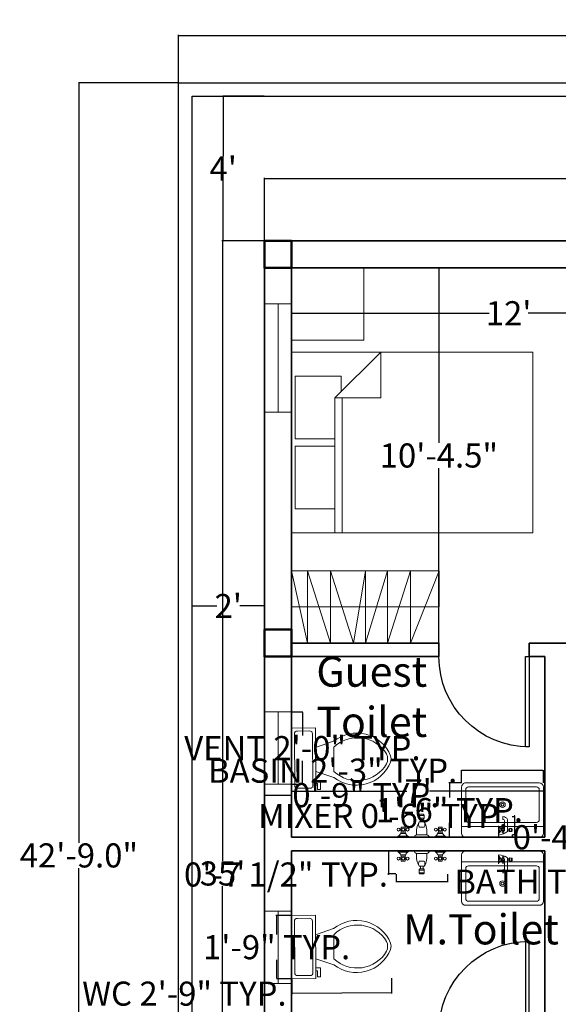
# Model space of a CAD drawing. Units: inches. Extents: x 20414 to 21627, y 49019 to 50314.
# Tile 6 of 10: x 20416 to 20594, y 49988 to 50314. Entities that reach past the tile are written whole.
import ezdxf

# ---------------------------------------------------------------- set-up
doc = ezdxf.new("R2010")
doc.units = ezdxf.units.IN
for name, color, linetype, lineweight in [('A-ANNO-DIMS', 7, 'Continuous', 18), ('A-AREA-IDEN', 7, 'Continuous', 18), ('A-FLOR-CASE', 2, 'Continuous', 18), ('C-PROP', 6, 'Continuous', 25), ('columns', 1, 'Continuous', 50), ('doors', 3, 'Continuous', 25), ('furniture', 2, 'Continuous', 18), ('plumbing', 1, 'Continuous', 18), ('walls', 6, 'Continuous', 35), ('windows', 3, 'Continuous', 18)]:
    doc.layers.add(name, color=color, linetype=linetype, lineweight=lineweight)
doc.styles.get("Standard").update_dxf_attribs({"font": 'arial.ttf'})
doc.dimstyles.get("Standard").update_dxf_attribs({"dimtxt": 8, "dimasz": 0.18, "dimexe": 0.18, "dimexo": 0.0625, "dimgap": 0.09, "dimtad": 0, "dimtih": 1, "dimtoh": 1, "dimdec": 1, "dimzin": 0, "dimdsep": 46, "dimlunit": 3, "dimtxsty": 'Standard', "dimcen": 0.09, "dimadec": 0, "dimazin": 0, "dimtfac": 1, "dimtdec": 1, "dimtofl": 0, "dimtmove": 0, "dimatfit": 3, "dimfxl": 1, "dimtolj": 1, "dimtzin": 0, "dimarcsym": 0})

# ---------------------------------------------------------------- blocks, each defined once
blk = doc.blocks.new('Bed - Queen')
for p, q in [((0, -80.00003), (0, 0)), ((0, 0), (59.99999, 0)), ((59.99999, 0), (59.99999, -80.00003)), ((7.99999, -1.2), (28.79998, -1.2)), ((7.99999, -14.4), (7.99999, -1.2)), ((28.79998, -1.2), (28.79998, -14.4)), ((31.19999, -1.2), (51.99999, -1.2)), ((31.19999, -14.4), (31.19999, -1.2)), ((51.99999, -1.2), (51.99999, -16.4)), ((0, -14.4), (44.8, -14.4)), ((59.99999, -29.6), (44.8, -14.4)), ((44.8, -14.4), (44.8, -29.6)), ((44.8, -16.8), (0, -16.8)), ((51.99999, -16.4), (46.79936, -16.4)), ((44.8, -29.6), (59.99999, -29.6)), ((59.99999, -80.00003), (0, -80.00003))]:
    blk.add_line(p, q)
blk = doc.blocks.new('Toilet - top')
for p, q in [((9.5, -6), (9.5, -2)), ((-10, -8.5), (-8, -8.5)), ((-10, -9.5), (-10, -8.5)), ((-7, -9.5), (-10, -9.5)), ((-8, -8.5), (-8, -8)), ((-7, -8), (-7, -9.5)), ((-4, -8), (-6, -14)), ((4, -8), (6, -14)), ((4, -14), (-4, -14))]:
    blk.add_line(p, q)
blk.add_lwpolyline([(10.5, -8), (10.5, 0), (-10.5, 0), (-10.5, -8)], close=True)
for points in [[(-9.5, -2), (-9.5, -6)], [(8.5, -1), (-8.5, -1)], [(-8.5, -7), (8.5, -7)]]:
    blk.add_lwpolyline(points)
for centre, radius, start, end in [((-8.62, -1.88), 0.884, 81.8699, 188.1301), ((8.62, -1.88), 0.884, 351.8699, 98.1301), ((-8.62, -6.12), 0.884, 171.8699, 278.1301), ((8.62, -6.12), 0.884, 261.8699, 8.1301), ((3.52, -21.58), 12.17, 141.4691, 247.9714), ((4.2, -21.82), 11.33, 136.3677, 238.9468), ((-3.52, -21.58), 12.17, 292.0284, 38.5307), ((-4.2, -21.82), 11.33, 301.053, 43.6321), ((0, -27.88), 4, 245.7318, 294.2682), ((0, -29), 4, 254.8605, 285.1395)]:
    blk.add_arc(centre, radius, start, end)
blk = doc.blocks.new('*U14')
for p, q in [((0, 0), (0, 6)), ((40, 0), (40, 6))]:
    blk.add_line(p, q)
blk.add_lwpolyline([(0, 0), (0, -40), (1.75, -40), (1.75, 0)], close=True)
blk.add_arc((0, 0), 40, 270, 0)
blk = doc.blocks.new('*U15')
for p, q in [((0, 0), (0, -6)), ((40, 0), (40, -6))]:
    blk.add_line(p, q)
blk.add_lwpolyline([(0, 0), (0, 40), (1.75, 40), (1.75, 0)], close=True)
blk.add_arc((0, 0), 40, 0, 90)
blk = doc.blocks.new('Faucet - Bathroom side')
for p, q in [((-0.625, 4.25), (0.375, 4.25)), ((0.375, 3.75), (-0.625, 3.75)), ((-0.375, 3), (-0.375, 3.5)), ((0.125, 3.5), (0.125, 3)), ((-1.625, 0), (-1.375, 0)), ((-1.375, 0), (1.375, 0)), ((-0.88366, 0.25), (0.88424, 0.25)), ((-0.625, 3), (3.375, 3)), ((-0.375, 1.625), (-0.625, 1.625)), ((-0.375, 1.375), (-0.625, 1.375)), ((0.48078, 0.75), (-0.47286, 0.75)), ((2.875, 2), (0.375, 2)), ((0.375, 1.625), (0.625, 1.625)), ((0.375, 1.375), (0.625, 1.375)), ((4.375, 1.5), (3.375, 1.5))]:
    blk.add_line(p, q)
for points in [[(-0.625, 3.75), (-0.625, 4.25)], [(-0.375, 4.5), (0.125, 4.5)], [(0.125, 3.5), (-0.375, 3.5)], [(0.375, 4.25), (0.375, 3.75)]]:
    blk.add_lwpolyline(points)
blk.add_lwpolyline([(-0.375, 1), (-0.375, 2), (0.375, 2), (0.375, 1)], close=True)
for centre in [(-0.875, 1.5), (0, 1.5), (0.875, 1.5)]:
    blk.add_circle(centre, 0.27951)
for centre, radius, start, end in [((-0.38253, 4.2575), 0.24259, 88.22243, 181.7776), ((-0.38253, 3.7424), 0.24259, 178.2224, 271.7776), ((0.13252, 4.2575), 0.24259, 358.2224, 91.77757), ((0.13252, 3.7424), 0.24259, 268.2224, 1.777565), ((3.45929, -0.0281), 5.08436, 143.4467, 179.6834), ((-1.75, 1.375), 1.42522, 285.2551, 344.7449), ((1.75, 1.375), 1.42522, 195.2551, 254.7449), ((-2.49562, -0.286), 3.38273, 9.709485, 29.48735), ((2.96867, 1.5936), 0.41699, 347.0192, 102.9808), ((2.70708, 1.4714), 1.66816, 0.9827695, 66.39737)]:
    blk.add_arc(centre, radius, start, end)
blk = doc.blocks.new('Sink-single - 30 in top')
blk.add_line((-15, -3.999996), (15, -3.999996))
for points in [[(-13.5, 0), (13.5, 0)], [(-15, -18.499996), (-15, -1.5)], [(15, -1.5), (15, -18.499996)], [(-13.5, -17.499996), (-13.5, -6.499996)], [(-12.5, -5.499996), (12.5, -5.499996)], [(13.5, -6.499996), (13.5, -17.499996)], [(13.5, -19.999996), (-13.5, -19.999996)], [(12.5, -18.499996), (-12.5, -18.499996)]]:
    blk.add_lwpolyline(points)
for radius in [1, 0.5]:
    blk.add_circle((0, -11.999996), radius)
for centre, radius, start, end in [((-13.5, -1.5), 1.5, 90, 180), ((13.5, -1.5), 1.5, 0, 90), ((-12.5, -6.499996), 1, 90, 180), ((12.5, -6.499996), 1, 0, 90), ((-12.5, -17.499996), 1, 180, 270), ((12.5, -17.499996), 1, 270, 0), ((-13.5, -18.499996), 1.5, 180, 270), ((13.5, -18.499996), 1.5, 270, 0)]:
    blk.add_arc(centre, radius, start, end)
blk = doc.blocks.new('Faucet - Bathroom front')
for p, q in [((-0.5, 4.25), (0.5, 4.25)), ((0.5, 3.75), (-0.5, 3.75)), ((-0.5, 3), (0.5, 3)), ((0.5, 2), (-0.5, 2)), ((-0.25, 3), (-0.25, 3.5)), ((0.25, 3.5), (0.25, 3)), ((-5, 0), (-2.25, 0)), ((-4.5087, 0.25), (-2.7408, 0.25)), ((-4, 1.625), (-4.25, 1.625)), ((-4, 1.375), (-4.25, 1.375)), ((-3.1442, 0.75), (-4.0979, 0.75)), ((-3.25, 1.625), (-3, 1.625)), ((-3.25, 1.375), (-3, 1.375)), ((-1.5, 0), (1.5, 0)), ((-1, 0.5), (1, 0.5)), ((2.25, 0), (5, 0)), ((2.7413, 0.25), (4.5092, 0.25)), ((3.25, 1.625), (3, 1.625)), ((3.25, 1.375), (3, 1.375)), ((4.1058, 0.75), (3.1521, 0.75)), ((4, 1.625), (4.25, 1.625)), ((4, 1.375), (4.25, 1.375))]:
    blk.add_line(p, q)
for points in [[(-0.5, 3.75), (-0.5, 4.25)], [(-0.25, 4.5), (0.25, 4.5)], [(0.5, 4.25), (0.5, 3.75)], [(0.25, 3.5), (-0.25, 3.5)]]:
    blk.add_lwpolyline(points)
for points in [[(-4, 1), (-4, 2), (-3.25, 2), (-3.25, 1)], [(3.25, 1), (3.25, 2), (4, 2), (4, 1)]]:
    blk.add_lwpolyline(points, close=True)
for centre in [(-4.5, 1.5), (-3.625, 1.5), (-2.75, 1.5), (2.75, 1.5), (3.625, 1.5), (4.5, 1.5)]:
    blk.add_circle(centre, 0.2795)
for centre, radius, start, end in [((-0.2575, 4.2575), 0.2426, 88.22243, 181.7776), ((0.2575, 4.2575), 0.2426, 358.2224, 91.77757), ((3, 1), 4.0311, 150.2551, 187.125), ((0.6413, 2.5), 1.246, 156.3417, 203.6583), ((-0.2575, 3.7425), 0.2426, 178.2224, 271.7776), ((0.2575, 3.7425), 0.2426, 268.2224, 1.777565), ((-3, 1), 4.0311, 352.875, 29.74488), ((-0.6413, 2.5), 1.246, 336.3417, 23.65835), ((-5.375, 1.375), 1.4252, 285.2551, 344.7449), ((-1.875, 1.375), 1.4252, 195.2551, 254.7449), ((-0.7962, -0.2038), 0.7327, 106.1502, 163.8498), ((0.7962, -0.2038), 0.7327, 16.1502, 73.84979), ((1.875, 1.375), 1.4252, 285.2551, 344.7449), ((5.375, 1.375), 1.4252, 195.2551, 254.7449)]:
    blk.add_arc(centre, radius, start, end)
blk = doc.blocks.new('*D29')
at = {"layer": 'A-ANNO-DIMS', "color": 0, "lineweight": -2, "transparency": 16777216}
for p, q in [((20506.01, 50219.94), (20506.01, 50216.8)), ((20649.99, 50219.94), (20649.99, 50216.8)), ((20506.19, 50216.98), (20571.5, 50216.98)), ((20649.81, 50216.98), (20584.5, 50216.98))]:
    blk.add_line(p, q, dxfattribs=at)
at = {"layer": 'A-ANNO-DIMS', "color": 0, "transparency": 16777216}
for points in [[(20506.19, 50217.01), (20506.19, 50216.95), (20506.01, 50216.98)], [(20649.81, 50217.01), (20649.81, 50216.95), (20649.99, 50216.98)]]:
    blk.add_solid(points, dxfattribs=at)
at = {"layer": 'Defpoints', "color": 0, "transparency": 16777216}
for p in [(20506.01, 50220.01), (20649.99, 50220.01), (20649.99, 50216.98)]:
    blk.add_point(p, dxfattribs=at)
at = {"layer": 'A-ANNO-DIMS', "color": 0, "transparency": 16777216, "insert": (20578, 50216.98), "char_height": 8, "attachment_point": 5}
blk.add_mtext("\\A1;12'", dxfattribs=at)
blk = doc.blocks.new('*D30')
at = {"layer": 'A-ANNO-DIMS', "color": 0, "lineweight": -2, "transparency": 16777216}
for p, q in [((20497.01, 50241.07), (20497.01, 50261.92)), ((20497.19, 50261.74), (20640.05, 50261.74)), ((20796.81, 50261.74), (20653.95, 50261.74)), ((20796.99, 50241.07), (20796.99, 50261.92))]:
    blk.add_line(p, q, dxfattribs=at)
at = {"layer": 'A-ANNO-DIMS', "color": 0, "transparency": 16777216}
for points in [[(20497.19, 50261.77), (20497.19, 50261.71), (20497.01, 50261.74)], [(20796.81, 50261.77), (20796.81, 50261.71), (20796.99, 50261.74)]]:
    blk.add_solid(points, dxfattribs=at)
at = {"layer": 'Defpoints', "color": 0, "transparency": 16777216}
for p in [(20796.99, 50261.74), (20497.01, 50241.01), (20796.99, 50241.01)]:
    blk.add_point(p, dxfattribs=at)
at = {"layer": 'A-ANNO-DIMS', "color": 0, "transparency": 16777216, "insert": (20647, 50261.74), "char_height": 8, "attachment_point": 5}
blk.add_mtext("\\A1;25'", dxfattribs=at)
blk = doc.blocks.new('*D31')
at = {"layer": 'A-ANNO-DIMS', "color": 0, "lineweight": -2, "transparency": 16777216}
for p, q in [((20496.94, 50241.01), (20482.91, 50241.01)), ((20483.09, 50240.83), (20483.09, 50035.18)), ((20483.09, 49821.19), (20483.09, 50026.83)), ((20496.93, 49821.01), (20482.91, 49821.01))]:
    blk.add_line(p, q, dxfattribs=at)
at = {"layer": 'A-ANNO-DIMS', "color": 0, "transparency": 16777216}
for points in [[(20483.06, 50240.83), (20483.12, 50240.83), (20483.09, 50241.01)], [(20483.06, 49821.19), (20483.12, 49821.19), (20483.09, 49821.01)]]:
    blk.add_solid(points, dxfattribs=at)
at = {"layer": 'Defpoints', "color": 0, "transparency": 16777216}
for p in [(20483.09, 50241.01), (20497.01, 50241.01), (20496.99, 49821.01)]:
    blk.add_point(p, dxfattribs=at)
at = {"layer": 'A-ANNO-DIMS', "color": 0, "transparency": 16777216, "insert": (20483.09, 50031.01), "char_height": 8, "attachment_point": 5}
blk.add_mtext("\\A1;35'", dxfattribs=at)
blk = doc.blocks.new('*D46')
at = {"layer": 'A-ANNO-DIMS', "color": 0, "lineweight": -2, "transparency": 16777216}
for p, q in [((20505.99, 50058.36), (20505.99, 50058.47)), ((20506.17, 50058.29), (20544.25, 50058.29)), ((20589.81, 50058.29), (20551.73, 50058.29)), ((20589.99, 50058.23), (20589.99, 50058.11))]:
    blk.add_line(p, q, dxfattribs=at)
at = {"layer": 'A-ANNO-DIMS', "color": 0, "transparency": 16777216}
for points in [[(20506.17, 50058.32), (20506.17, 50058.26), (20505.99, 50058.29)], [(20589.81, 50058.32), (20589.81, 50058.26), (20589.99, 50058.29)]]:
    blk.add_solid(points, dxfattribs=at)
at = {"layer": 'Defpoints', "color": 0, "transparency": 16777216}
for p in [(20505.99, 50058.29), (20589.99, 50058.29), (20589.99, 50058.29)]:
    blk.add_point(p, dxfattribs=at)
at = {"layer": 'A-ANNO-DIMS', "color": 0, "transparency": 16777216, "insert": (20547.99, 50058.29), "char_height": 8, "attachment_point": 5}
blk.add_mtext("\\A1;7'", dxfattribs=at)
blk = doc.blocks.new('*D53')
at = {"layer": 'A-ANNO-DIMS', "color": 0, "lineweight": -2, "transparency": 16777216}
for p, q in [((20554.86, 50231.83), (20554.86, 50173.93)), ((20554.92, 50232.01), (20555.04, 50232.01)), ((20554.86, 50107.69), (20554.86, 50165.58)), ((20554.92, 50107.51), (20555.04, 50107.51))]:
    blk.add_line(p, q, dxfattribs=at)
at = {"layer": 'A-ANNO-DIMS', "color": 0, "transparency": 16777216}
for points in [[(20554.83, 50231.83), (20554.89, 50231.83), (20554.86, 50232.01)], [(20554.83, 50107.69), (20554.89, 50107.69), (20554.86, 50107.51)]]:
    blk.add_solid(points, dxfattribs=at)
at = {"layer": 'Defpoints', "color": 0, "transparency": 16777216}
for p in [(20554.86, 50232.01), (20554.86, 50232.01), (20554.86, 50107.51)]:
    blk.add_point(p, dxfattribs=at)
at = {"layer": 'A-ANNO-DIMS', "color": 0, "transparency": 16777216, "insert": (20554.86, 50169.76), "char_height": 8, "attachment_point": 5}
blk.add_mtext('\\A1;10\'-4.5"', dxfattribs=at)
blk = doc.blocks.new('*D60')
at = {"layer": 'A-ANNO-DIMS', "color": 0, "lineweight": -2, "transparency": 16777216}
for p, q in [((20468.43, 50293.51), (20435.25, 50293.51)), ((20435.43, 50293.33), (20435.43, 50041.18)), ((20435.43, 49780.69), (20435.43, 50032.83)), ((20468.43, 49780.51), (20435.25, 49780.51))]:
    blk.add_line(p, q, dxfattribs=at)
at = {"layer": 'A-ANNO-DIMS', "color": 0, "transparency": 16777216}
for points in [[(20435.4, 50293.33), (20435.46, 50293.33), (20435.43, 50293.51)], [(20435.4, 49780.69), (20435.46, 49780.69), (20435.43, 49780.51)]]:
    blk.add_solid(points, dxfattribs=at)
at = {"layer": 'Defpoints', "color": 0, "transparency": 16777216}
for p in [(20468.49, 50293.51), (20435.43, 49780.51), (20468.49, 49780.51)]:
    blk.add_point(p, dxfattribs=at)
at = {"layer": 'A-ANNO-DIMS', "color": 0, "transparency": 16777216, "insert": (20435.43, 50037.01), "char_height": 8, "attachment_point": 5}
blk.add_mtext('\\A1;42\'-9.0"', dxfattribs=at)
blk = doc.blocks.new('*D61')
at = {"layer": 'A-ANNO-DIMS', "color": 0, "lineweight": -2, "transparency": 16777216}
for p, q in [((20468.49, 50293.57), (20468.49, 50309.35)), ((20468.67, 50309.17), (20688.5, 50309.17)), ((20945.31, 50309.17), (20725.48, 50309.17)), ((20945.49, 50293.57), (20945.49, 50309.35))]:
    blk.add_line(p, q, dxfattribs=at)
at = {"layer": 'A-ANNO-DIMS', "color": 0, "transparency": 16777216}
for points in [[(20468.67, 50309.2), (20468.67, 50309.14), (20468.49, 50309.17)], [(20945.31, 50309.2), (20945.31, 50309.14), (20945.49, 50309.17)]]:
    blk.add_solid(points, dxfattribs=at)
at = {"layer": 'Defpoints', "color": 0, "transparency": 16777216}
for p in [(20945.49, 50309.17), (20468.49, 50293.51), (20945.49, 50293.51)]:
    blk.add_point(p, dxfattribs=at)
at = {"layer": 'A-ANNO-DIMS', "color": 0, "transparency": 16777216, "insert": (20706.99, 50309.17), "char_height": 8, "attachment_point": 5}
blk.add_mtext('\\A1;39\'-9.0"', dxfattribs=at)
blk = doc.blocks.new('*D62')
at = {"layer": 'A-ANNO-DIMS', "color": 0, "lineweight": -2, "transparency": 16777216}
for p, q in [((20496.94, 50289.01), (20483.14, 50289.01)), ((20483.32, 50288.83), (20483.32, 50269.1)), ((20483.32, 50241.19), (20483.32, 50260.92)), ((20496.94, 50241.01), (20483.14, 50241.01))]:
    blk.add_line(p, q, dxfattribs=at)
at = {"layer": 'A-ANNO-DIMS', "color": 0, "transparency": 16777216}
for points in [[(20483.29, 50288.83), (20483.35, 50288.83), (20483.32, 50289.01)], [(20483.29, 50241.19), (20483.35, 50241.19), (20483.32, 50241.01)]]:
    blk.add_solid(points, dxfattribs=at)
at = {"layer": 'Defpoints', "color": 0, "transparency": 16777216}
for p in [(20483.32, 50289.01), (20497.01, 50289.01), (20497.01, 50241.01)]:
    blk.add_point(p, dxfattribs=at)
at = {"layer": 'A-ANNO-DIMS', "color": 0, "transparency": 16777216, "insert": (20483.32, 50265.01), "char_height": 8, "attachment_point": 5}
blk.add_mtext("\\A1;4'", dxfattribs=at)
blk = doc.blocks.new('*D64')
at = {"layer": 'A-ANNO-DIMS', "color": 0, "lineweight": -2, "transparency": 16777216}
for p, q in [((20472.99, 50112.07), (20472.99, 50119.98)), ((20473.17, 50119.8), (20481.15, 50119.8)), ((20496.81, 50119.8), (20488.83, 50119.8)), ((20496.99, 50112.07), (20496.99, 50119.98))]:
    blk.add_line(p, q, dxfattribs=at)
at = {"layer": 'A-ANNO-DIMS', "color": 0, "transparency": 16777216}
for points in [[(20473.17, 50119.83), (20473.17, 50119.77), (20472.99, 50119.8)], [(20496.81, 50119.83), (20496.81, 50119.77), (20496.99, 50119.8)]]:
    blk.add_solid(points, dxfattribs=at)
at = {"layer": 'Defpoints', "color": 0, "transparency": 16777216}
for p in [(20472.99, 50119.8), (20472.99, 50112.01), (20496.99, 50112.01)]:
    blk.add_point(p, dxfattribs=at)
at = {"layer": 'A-ANNO-DIMS', "color": 0, "transparency": 16777216, "insert": (20484.99, 50119.8), "char_height": 8, "attachment_point": 5}
blk.add_mtext("\\A1;2'", dxfattribs=at)
blk = doc.blocks.new('WINDOW-36IN-PLAN')
for p, q in [((9, 36), (0, 36)), ((4.5, 36), (4.5, 0)), ((9, 0), (0, 0))]:
    blk.add_line(p, q)
blk = doc.blocks.new('VENT-24IN-PLAN')
for p, q in [((9, 24), (0, 24)), ((4.5, 0), (4.5, 24)), ((9, 0), (0, 0))]:
    blk.add_line(p, q)
blk = doc.blocks.new('COLUMN-9X9')
blk.add_lwpolyline([(0, 9), (0, 0), (9, 0), (9, 9), (0, 9)])
blk = doc.blocks.new('NIGHTSTAND-24IN')
blk.add_lwpolyline([(0, 0), (0, 24), (24, 24), (24, 0), (0, 0)])
blk = doc.blocks.new('WARDROBE-49IN')
for q in [(0, 24), (48.87, 0)]:
    blk.add_line((49, 24), q)
blk.add_lwpolyline([(0, 24), (5.3, 0), (5.3, 24), (12.93, 0), (12.93, 24), (20.56, 0), (24.5, 24), (24.5, 0), (31.88, 24), (31.88, 0), (39.51, 24), (39.51, 0), (49, 24), (48.94, 12), (0, 12)])
blk = doc.blocks.new('*D86')
at = {"layer": 'A-ANNO-DIMS', "color": 0, "lineweight": -2, "transparency": 16777216}
for p, q in [((20506.05, 50084.62), (20509.77, 50084.62)), ((20509.59, 50084.44), (20509.59, 50076.79)), ((20509.59, 50060.8), (20509.59, 50068.44)), ((20506.05, 50060.62), (20509.77, 50060.62))]:
    blk.add_line(p, q, dxfattribs=at)
at = {"layer": 'A-ANNO-DIMS', "color": 0, "transparency": 16777216}
for points in [[(20509.56, 50084.44), (20509.62, 50084.44), (20509.59, 50084.62)], [(20509.56, 50060.8), (20509.62, 50060.8), (20509.59, 50060.62)]]:
    blk.add_solid(points, dxfattribs=at)
at = {"layer": 'Defpoints', "color": 0, "transparency": 16777216}
for p in [(20505.99, 50084.62), (20509.59, 50084.62), (20505.99, 50060.62)]:
    blk.add_point(p, dxfattribs=at)
at = {"layer": 'A-ANNO-DIMS', "color": 0, "transparency": 16777216, "insert": (20509.59, 50072.62), "char_height": 8, "attachment_point": 5}
blk.add_mtext('\\A1;VENT 2\'-0" TYP.', dxfattribs=at)
blk = doc.blocks.new('*D87')
at = {"layer": 'A-ANNO-DIMS', "color": 0, "lineweight": -2, "transparency": 16777216}
for p, q in [((20496.99, 50060.55), (20496.99, 50056.84)), ((20505.99, 50060.55), (20505.99, 50056.84)), ((20497.17, 50057.02), (20505.81, 50057.02)), ((20505.99, 50057.02), (20506.17, 50057.02))]:
    blk.add_line(p, q, dxfattribs=at)
at = {"layer": 'A-ANNO-DIMS', "color": 0, "transparency": 16777216}
for points in [[(20497.17, 50057.05), (20497.17, 50056.99), (20496.99, 50057.02)], [(20505.81, 50057.05), (20505.81, 50056.99), (20505.99, 50057.02)]]:
    blk.add_solid(points, dxfattribs=at)
at = {"layer": 'Defpoints', "color": 0, "transparency": 16777216}
for p in [(20496.99, 50060.62), (20505.99, 50060.62), (20505.99, 50057.02)]:
    blk.add_point(p, dxfattribs=at)
at = {"layer": 'A-ANNO-DIMS', "color": 0, "transparency": 16777216, "insert": (20530.64, 50057.02), "char_height": 8, "attachment_point": 5}
blk.add_mtext('\\A1;0\'-9" TYP.', dxfattribs=at)
blk = doc.blocks.new('*D90')
at = {"layer": 'A-ANNO-DIMS', "color": 0, "lineweight": -2, "transparency": 16777216}
for p, q in [((20539.12, 49996.29), (20539.16, 49991.22)), ((20506.07, 49996.03), (20506.11, 49990.96)), ((20506.11, 49991.14), (20505.93, 49991.13)), ((20538.98, 49991.39), (20506.29, 49991.14))]:
    blk.add_line(p, q, dxfattribs=at)
at = {"layer": 'A-ANNO-DIMS', "color": 0, "transparency": 16777216}
for points in [[(20506.29, 49991.17), (20506.29, 49991.11), (20506.11, 49991.14)], [(20538.98, 49991.42), (20538.98, 49991.36), (20539.16, 49991.4)]]:
    blk.add_solid(points, dxfattribs=at)
at = {"layer": 'Defpoints', "color": 0, "transparency": 16777216}
for p in [(20539.12, 49996.35), (20506.07, 49996.09), (20506.11, 49991.14)]:
    blk.add_point(p, dxfattribs=at)
at = {"layer": 'A-ANNO-DIMS', "color": 0, "transparency": 16777216, "insert": (20470.43, 49991.13), "char_height": 8, "attachment_point": 5}
blk.add_mtext('\\A1;WC 2\'-9" TYP.', dxfattribs=at)
blk = doc.blocks.new('*D91')
at = {"layer": 'A-ANNO-DIMS', "color": 0, "lineweight": -2, "transparency": 16777216}
for p, q in [((20505.85, 50017.09), (20500.77, 50017.05)), ((20500.95, 50016.87), (20501, 50010.73)), ((20501.12, 49996.23), (20501.07, 50002.38)), ((20506.01, 49996.09), (20500.94, 49996.05))]:
    blk.add_line(p, q, dxfattribs=at)
at = {"layer": 'A-ANNO-DIMS', "color": 0, "transparency": 16777216}
for points in [[(20500.98, 50016.87), (20500.92, 50016.87), (20500.95, 50017.05)], [(20501.15, 49996.23), (20501.09, 49996.23), (20501.12, 49996.05)]]:
    blk.add_solid(points, dxfattribs=at)
at = {"layer": 'Defpoints', "color": 0, "transparency": 16777216}
for p in [(20500.95, 50017.05), (20505.91, 50017.09), (20506.07, 49996.09)]:
    blk.add_point(p, dxfattribs=at)
at = {"layer": 'A-ANNO-DIMS', "color": 0, "transparency": 16777216, "insert": (20501.03, 50006.55), "char_height": 8, "attachment_point": 5}
blk.add_mtext('\\A1;1\'-9" TYP.', dxfattribs=at)
blk = doc.blocks.new('*D92')
at = {"layer": 'A-ANNO-DIMS', "color": 0, "lineweight": -2, "transparency": 16777216}
for p, q in [((20579.17, 50049.94), (20580.19, 50049.95)), ((20580.01, 50050.13), (20579.83, 50050.13)), ((20580.01, 50049.95), (20580.01, 50050.13)), ((20580.09, 50044.13), (20580.01, 50049.77)), ((20579.25, 50043.94), (20580.27, 50043.95))]:
    blk.add_line(p, q, dxfattribs=at)
at = {"layer": 'A-ANNO-DIMS', "color": 0, "transparency": 16777216}
for points in [[(20580.04, 50049.77), (20579.98, 50049.77), (20580.01, 50049.95)], [(20580.12, 50044.13), (20580.06, 50044.13), (20580.09, 50043.95)]]:
    blk.add_solid(points, dxfattribs=at)
at = {"layer": 'Defpoints', "color": 0, "transparency": 16777216}
for p in [(20579.11, 50049.94), (20580.01, 50049.95), (20579.19, 50043.94)]:
    blk.add_point(p, dxfattribs=at)
at = {"layer": 'A-ANNO-DIMS', "color": 0, "transparency": 16777216, "insert": (20536.29, 50050.13), "char_height": 8, "attachment_point": 5}
blk.add_mtext('\\A1;MIXER 0\'-6" TYP.', dxfattribs=at)
blk = doc.blocks.new('*D93')
at = {"layer": 'A-ANNO-DIMS', "color": 0, "lineweight": -2, "transparency": 16777216}
for p, q in [((20574.69, 50043.81), (20574.71, 50042.8)), ((20574.88, 50042.98), (20579.02, 50043.04)), ((20579.19, 50043.88), (20579.21, 50042.86)), ((20579.2, 50043.04), (20579.38, 50043.04))]:
    blk.add_line(p, q, dxfattribs=at)
at = {"layer": 'A-ANNO-DIMS', "color": 0, "transparency": 16777216}
for points in [[(20574.88, 50043.01), (20574.88, 50042.95), (20574.7, 50042.98)], [(20579.02, 50043.07), (20579.02, 50043.01), (20579.2, 50043.04)]]:
    blk.add_solid(points, dxfattribs=at)
at = {"layer": 'Defpoints', "color": 0, "transparency": 16777216}
for p in [(20574.69, 50043.88), (20579.19, 50043.94), (20579.2, 50043.04)]:
    blk.add_point(p, dxfattribs=at)
at = {"layer": 'A-ANNO-DIMS', "color": 0, "transparency": 16777216, "insert": (20613.18, 50043.04), "char_height": 8, "attachment_point": 5}
blk.add_mtext('\\A1;0\'-4 1/2" TYP.', dxfattribs=at)
blk = doc.blocks.new('*D94')
at = {"layer": 'A-ANNO-DIMS', "color": 0, "lineweight": -2, "transparency": 16777216}
for p, q in [((20562.42, 50065.14), (20562.24, 50065.14)), ((20562.42, 50061.14), (20562.42, 50065.32)), ((20589.35, 50065.14), (20562.6, 50065.14)), ((20589.53, 50061.14), (20589.53, 50065.32))]:
    blk.add_line(p, q, dxfattribs=at)
at = {"layer": 'A-ANNO-DIMS', "color": 0, "transparency": 16777216}
for points in [[(20562.6, 50065.17), (20562.6, 50065.11), (20562.42, 50065.14)], [(20589.35, 50065.17), (20589.35, 50065.11), (20589.53, 50065.14)]]:
    blk.add_solid(points, dxfattribs=at)
at = {"layer": 'Defpoints', "color": 0, "transparency": 16777216}
for p in [(20562.42, 50065.14), (20562.42, 50061.08), (20589.53, 50061.08)]:
    blk.add_point(p, dxfattribs=at)
at = {"layer": 'A-ANNO-DIMS', "color": 0, "transparency": 16777216, "insert": (20519.62, 50065.14), "char_height": 8, "attachment_point": 5}
blk.add_mtext('\\A1;BASIN 2\'-3" TYP.', dxfattribs=at)
blk = doc.blocks.new('*D95')
at = {"layer": 'A-ANNO-DIMS', "color": 0, "lineweight": -2, "transparency": 16777216}
for p, q in [((20562.35, 50061.08), (20558.17, 50061.08)), ((20558.35, 50060.9), (20558.35, 50056.22)), ((20558.35, 50043.19), (20558.35, 50047.87)), ((20562.35, 50043.01), (20558.17, 50043.01))]:
    blk.add_line(p, q, dxfattribs=at)
at = {"layer": 'A-ANNO-DIMS', "color": 0, "transparency": 16777216}
for points in [[(20558.32, 50060.9), (20558.38, 50060.9), (20558.35, 50061.08)], [(20558.32, 50043.19), (20558.38, 50043.19), (20558.35, 50043.01)]]:
    blk.add_solid(points, dxfattribs=at)
at = {"layer": 'Defpoints', "color": 0, "transparency": 16777216}
for p in [(20562.42, 50061.08), (20558.35, 50043.01), (20562.42, 50043.01)]:
    blk.add_point(p, dxfattribs=at)
at = {"layer": 'A-ANNO-DIMS', "color": 0, "transparency": 16777216, "insert": (20558.35, 50052.04), "char_height": 8, "attachment_point": 5}
blk.add_mtext('\\A1;1\'-6" TYP.', dxfattribs=at)
blk = doc.blocks.new('*D96')
at = {"layer": 'A-ANNO-DIMS', "color": 0, "lineweight": -2, "transparency": 16777216}
for p, q in [((20540.67, 50030.79), (20540.67, 50028.12)), ((20557.68, 50030.79), (20557.68, 50028.12)), ((20540.85, 50028.3), (20557.5, 50028.3)), ((20557.68, 50028.3), (20557.86, 50028.3))]:
    blk.add_line(p, q, dxfattribs=at)
at = {"layer": 'A-ANNO-DIMS', "color": 0, "transparency": 16777216}
for points in [[(20540.85, 50028.33), (20540.85, 50028.27), (20540.67, 50028.3)], [(20557.5, 50028.33), (20557.5, 50028.27), (20557.68, 50028.3)]]:
    blk.add_solid(points, dxfattribs=at)
at = {"layer": 'Defpoints', "color": 0, "transparency": 16777216}
for p in [(20540.67, 50030.85), (20557.68, 50030.85), (20557.68, 50028.3)]:
    blk.add_point(p, dxfattribs=at)
at = {"layer": 'A-ANNO-DIMS', "color": 0, "transparency": 16777216, "insert": (20611.03, 50028.3), "char_height": 8, "attachment_point": 5}
blk.add_mtext('\\A1;BATH TAP 1\'-5" TYP.', dxfattribs=at)
blk = doc.blocks.new('*D97')
at = {"layer": 'A-ANNO-DIMS', "color": 0, "lineweight": -2, "transparency": 16777216}
for p, q in [((20540.6, 50038.51), (20537.93, 50038.51)), ((20538.11, 50038.33), (20538.11, 50031.03)), ((20540.6, 50030.85), (20537.93, 50030.85)), ((20538.11, 50030.67), (20537.93, 50030.67)), ((20538.11, 50030.85), (20538.11, 50030.67))]:
    blk.add_line(p, q, dxfattribs=at)
at = {"layer": 'A-ANNO-DIMS', "color": 0, "transparency": 16777216}
for points in [[(20538.08, 50038.33), (20538.14, 50038.33), (20538.11, 50038.51)], [(20538.08, 50031.03), (20538.14, 50031.03), (20538.11, 50030.85)]]:
    blk.add_solid(points, dxfattribs=at)
at = {"layer": 'Defpoints', "color": 0, "transparency": 16777216}
for p in [(20540.67, 50038.51), (20538.11, 50030.85), (20540.67, 50030.85)]:
    blk.add_point(p, dxfattribs=at)
at = {"layer": 'A-ANNO-DIMS', "color": 0, "transparency": 16777216, "insert": (20504.14, 50030.67), "char_height": 8, "attachment_point": 5}
blk.add_mtext('\\A1;0\'-7 1/2" TYP.', dxfattribs=at)

msp = doc.modelspace()

# ---------------------------------------------------------------- linework, layer by layer
at = {"layer": 'C-PROP'}
for p, q in [((20468.49, 49780.51), (20468.49, 50293.51)), ((20468.49, 50293.51), (20945.49, 50293.51)), ((20472.99, 49785.01), (20472.99, 50289.01)), ((20472.99, 50289.01), (20940.99, 50289.01))]:
    msp.add_line(p, q, dxfattribs=at)
at = {"layer": 'walls'}
for p, q in [((20496.99, 49821.01), (20496.99, 50241.01)), ((20496.99, 50241.01), (20796.99, 50241.01)), ((20505.99, 50232.01), (20649.99, 50232.01)), ((20505.99, 50107.51), (20505.99, 50232.01)), ((20554.86, 50107.51), (20505.99, 50107.51)), ((20554.86, 50107.51), (20554.86, 50103.01)), ((20584.86, 50107.51), (20584.86, 50103.01)), ((20604.99, 50107.51), (20584.86, 50107.51)), ((20554.86, 50103.01), (20505.99, 50103.01)), ((20505.99, 50043.01), (20505.99, 50103.01)), ((20589.99, 50103.01), (20584.86, 50103.01)), ((20589.99, 50043.01), (20589.99, 50103.01)), ((20589.99, 50043.01), (20505.99, 50043.01)), ((20589.99, 50038.51), (20505.99, 50038.51)), ((20505.99, 49978.51), (20505.99, 50038.51)), ((20589.99, 49978.51), (20589.99, 50038.51))]:
    msp.add_line(p, q, dxfattribs=at)

# ---------------------------------------------------------------- block references
at = {"layer": 'A-FLOR-CASE'}
msp.add_blockref('WARDROBE-49IN', (20505.99, 50107.51), dxfattribs=at)
at = {"layer": 'columns'}
for p in [(20497.01, 50232.01), (20496.99, 50103.01)]:
    msp.add_blockref('COLUMN-9X9', p, dxfattribs=at)
at = {"layer": 'doors', "xscale": -0.75, "yscale": 0.75, "zscale": 0.75}
for name, p in [('*U14', (20584.86, 50103.01)), ('*U15', (20584.86, 49978.51))]:
    msp.add_blockref(name, p, dxfattribs=at)
at = {"layer": 'furniture'}
msp.add_blockref('NIGHTSTAND-24IN', (20506.01, 50208.01), dxfattribs=at)
at = {"layer": 'furniture', "rotation": 90}
msp.add_blockref('Bed - Queen', (20505.99, 50144.1), dxfattribs=at)
at = {"layer": 'plumbing'}
for name, p, rotation in [('Toilet - top', (20505.99, 50068.79), 90.45084889114678), ('Faucet - Bathroom side', (20574.67, 50035.58), 269.196606704899), ('Toilet - top', (20505.99, 50006.59), 90.45084889114678)]:
    msp.add_blockref(name, p, dxfattribs=dict(at, rotation=rotation))
at = {"layer": 'plumbing', "rotation": 180}
for name, p, xscale, yscale, zscale in [('Sink-single - 30 in top', (20575.97, 50043.01), 0.9035913028591334, 0.9035913028591334, 0.9035913028591334), ('Faucet - Bathroom front', (20549.17, 50038.51), -1.701154593653001, 1.701154593653001, 1.701154593653001)]:
    msp.add_blockref(name, p, dxfattribs=dict(at, xscale=xscale, yscale=yscale, zscale=zscale))
at = {"layer": 'plumbing'}
for name, p, xscale, yscale, zscale in [('Faucet - Bathroom front', (20549.17, 50043.01), 1.701154593653001, 1.701154593653001, 1.701154593653001), ('Sink-single - 30 in top', (20575.97, 50038.51), -0.9035913028591334, 0.9035913028591334, 0.9035913028591334)]:
    msp.add_blockref(name, p, dxfattribs=dict(at, xscale=xscale, yscale=yscale, zscale=zscale))
at = {"layer": 'plumbing', "xscale": -1, "rotation": 270.803393295101}
msp.add_blockref('Faucet - Bathroom side', (20574.67, 50045.5), dxfattribs=at)
at = {"layer": 'windows', "rotation": 180}
msp.add_blockref('WINDOW-36IN-PLAN', (20505.99, 50220.13), dxfattribs=at)
at = {"layer": 'windows'}
for p in [(20496.99, 50060.62), (20496.99, 49994.53)]:
    msp.add_blockref('VENT-24IN-PLAN', p, dxfattribs=at)

# ---------------------------------------------------------------- texts
at = {"layer": 'A-AREA-IDEN', "char_height": 10, "attachment_point": 1}
for s, width, heights, insert in [('Guest\\PToilet', 43.1663, [28.71], (20514.21, 50103.01)), ('M.Toilet', 44.4717, [34.97], (20543.02, 50017.47))]:
    msp.add_mtext_dynamic_manual_height_columns(s, width=width, gutter_width=50, heights=heights, dxfattribs=dict(at, insert=insert))

# ---------------------------------------------------------------- dimensions: what is measured, and where the dimension line sits
at = {"layer": 'A-ANNO-DIMS'}
for base, p1, p2, picture, middle in [((20945.49, 50309.17), (20468.49, 50293.51), (20945.49, 50293.51), '*D61', (20706.99, 50309.17)), ((20796.99, 50261.74), (20497.01, 50241.01), (20796.99, 50241.01), '*D30', (20647, 50261.74)), ((20649.99, 50216.98), (20506.01, 50220.01), (20649.99, 50220.01), '*D29', (20578, 50216.98)), ((20472.99, 50119.8), (20496.99, 50112.01), (20472.99, 50112.01), '*D64', (20484.99, 50119.8)), ((20589.99, 50058.29), (20505.99, 50058.29), (20589.99, 50058.29), '*D46', (20547.99, 50058.29))]:
    dim = msp.add_linear_dim(base=base, p1=p1, p2=p2, dimstyle='Standard', override={"dimclrd": 0, "dimclre": 0, "dimclrt": 0}, dxfattribs=at)
    dim.commit()
    dim.dimension.update_dxf_attribs({"geometry": picture, "text_midpoint": middle})
for base, p1, p2, picture, middle in [((20435.43, 49780.51), (20468.49, 50293.51), (20468.49, 49780.51), '*D60', (20435.43, 50037.01)), ((20483.32, 50289.01), (20497.01, 50241.01), (20497.01, 50289.01), '*D62', (20483.32, 50265.01)), ((20483.09, 50241.01), (20496.99, 49821.01), (20497.01, 50241.01), '*D31', (20483.09, 50031.01)), ((20554.86, 50232.01), (20554.86, 50107.51), (20554.86, 50232.01), '*D53', (20554.86, 50169.76))]:
    dim = msp.add_linear_dim(base=base, p1=p1, p2=p2, angle=90, dimstyle='Standard', override={"dimclrd": 0, "dimclre": 0, "dimclrt": 0}, dxfattribs=at)
    dim.commit()
    dim.dimension.update_dxf_attribs({"geometry": picture, "text_midpoint": middle})
for base, p1, p2, angle, text, picture, middle in [((20509.59, 50084.62), (20505.99, 50060.62), (20505.99, 50084.62), 90, 'VENT <> TYP.', '*D86', (20509.59, 50072.62)), ((20562.42, 50065.14), (20589.53, 50061.08), (20562.42, 50061.08), 180, 'BASIN <> TYP.', '*D94', (20519.62, 50065.14)), ((20580.01, 50049.95), (20579.19, 50043.94), (20579.11, 50049.94), 90.8034, 'MIXER <> TYP.', '*D92', (20536.29, 50050.13)), ((20558.35, 50043.01), (20562.42, 50061.08), (20562.42, 50043.01), 270, '<> TYP.', '*D95', (20558.35, 50052.04)), ((20579.2, 50043.04), (20574.69, 50043.88), (20579.19, 50043.94), 0.8034, '<> TYP.', '*D93', (20613.18, 50043.04)), ((20538.11, 50030.85), (20540.67, 50038.51), (20540.67, 50030.85), 270, '<> TYP.', '*D97', (20504.14, 50030.67)), ((20500.95, 50017.05), (20506.07, 49996.09), (20505.91, 50017.09), 90.4508, '<> TYP.', '*D91', (20501.03, 50006.55)), ((20506.1127, 49991.1352), (20539.1189, 49996.352), (20506.0737, 49996.092), 180.4508, 'WC <> TYP.', '*D90', (20470.4348, 49991.1338))]:
    dim = msp.add_linear_dim(base=base, p1=p1, p2=p2, angle=angle, text=text, dimstyle='Standard', override={"dimdec": 1, "dimlfac": 1, "dimrnd": 0, "dimzin": 1, "dimdsep": 46, "dimlunit": 4, "dimfrac": 2}, dxfattribs=at)
    dim.commit()
    dim.dimension.update_dxf_attribs({"geometry": picture, "text_midpoint": middle})
for base, p1, p2, text, picture, middle in [((20505.99, 50057.02), (20496.99, 50060.62), (20505.99, 50060.62), '<> TYP.', '*D87', (20530.64, 50057.02)), ((20557.68, 50028.3), (20540.67, 50030.85), (20557.68, 50030.85), 'BATH TAP <> TYP.', '*D96', (20611.03, 50028.3))]:
    dim = msp.add_linear_dim(base=base, p1=p1, p2=p2, text=text, dimstyle='Standard', override={"dimdec": 1, "dimlfac": 1, "dimrnd": 0, "dimzin": 1, "dimdsep": 46, "dimlunit": 4, "dimfrac": 2}, dxfattribs=at)
    dim.commit()
    dim.dimension.update_dxf_attribs({"geometry": picture, "text_midpoint": middle})

doc.saveas('drawing.dxf')
